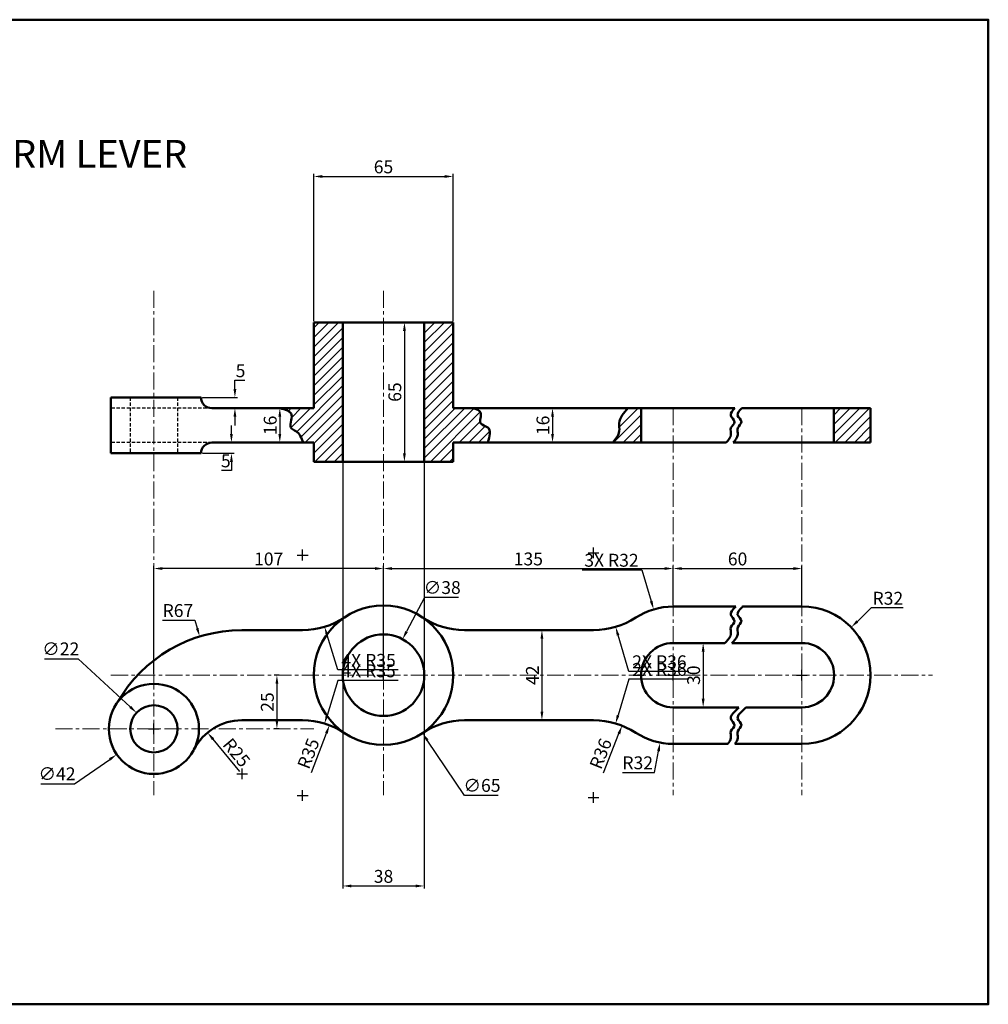
# Model space of a CAD drawing. Units: millimetres. Extents: x -1099 to -222, y 37 to 495.
# Tile 3 of 3: x -674 to -222, y 37 to 495. Entities that reach past the tile are written whole.
import ezdxf

# ---------------------------------------------------------------- set-up
doc = ezdxf.new("R2010")
doc.units = ezdxf.units.MM
doc.header["$LTSCALE"] = 0.5
doc.linetypes.add('CENTER', pattern=[50.8, 31.75, -6.35, 6.35, -6.35])
doc.linetypes.add('HIDDEN', pattern=[9.525, 6.35, -3.175])
for name, color, linetype, lineweight in [('M-CNTR', 1, 'CENTER', 18), ('M-DIMS', 2, 'Continuous', 25), ('M-HATC', 8, 'Continuous', 18), ('M-HIDN', 4, 'HIDDEN', 25), ('M-OUTL', 7, 'Continuous', 50), ('M-TEXT', 7, 'Continuous', 25), ('M-TTLB', 7, 'Continuous', 50)]:
    doc.layers.add(name, color=color, linetype=linetype, lineweight=lineweight)
doc.styles.get("Standard").update_dxf_attribs({"font": 'arial.ttf'})
doc.dimstyles.new('ISO-25', dxfattribs={"dimtxt": 6, "dimasz": 4, "dimexe": 1.25, "dimexo": 0.625, "dimtad": 1, "dimtoh": 1, "dimtxsty": 'Standard', "dimcen": 2.5, "dimadec": 0, "dimazin": 0, "dimtfac": 1, "dimtofl": 0, "dimtmove": 0, "dimatfit": 3, "dimfxl": 1, "dimarcsym": 0})
pattern_1 = [(45, (-1406.9138, -374.9262), (-2.245064, 2.245064), [])]

# ---------------------------------------------------------------- blocks, each defined once
blk = doc.blocks.new('*D20')
at = {"layer": 'Defpoints', "color": 0, "ltscale": 0.5, "transparency": 16777216}
for p in [(-589.05, 319.35), (-573.3, 319.35), (-584.25, 314.35)]:
    blk.add_point(p, dxfattribs=at)
at = {"layer": 'M-DIMS', "color": 0, "lineweight": -2, "ltscale": 0.5, "transparency": 16777216}
for p, q in [((-573.3, 323.35), (-573.3, 327.35)), ((-573.3, 327.35), (-568.69, 327.35)), ((-588.42, 319.35), (-572.05, 319.35)), ((-583.62, 314.35), (-572.05, 314.35)), ((-573.3, 310.35), (-573.3, 306.35))]:
    blk.add_line(p, q, dxfattribs=at)
at = {"layer": 'M-DIMS', "color": 0, "ltscale": 0.5, "transparency": 16777216}
for points in [[(-573.96, 323.35), (-572.63, 323.35), (-573.3, 319.35)], [(-573.96, 310.35), (-572.63, 310.35), (-573.3, 314.35)]]:
    blk.add_solid(points, dxfattribs=at)
at = {"layer": 'M-DIMS', "color": 0, "ltscale": 0.5, "transparency": 16777216, "insert": (-570.68, 331.02), "char_height": 6, "attachment_point": 5}
blk.add_mtext('5', dxfattribs=at)
blk = doc.blocks.new('*D21')
at = {"layer": 'Defpoints', "color": 0, "ltscale": 0.5, "transparency": 16777216}
for p in [(-584.05, 298.35), (-574.92, 298.35), (-589.05, 293.35)]:
    blk.add_point(p, dxfattribs=at)
at = {"layer": 'M-DIMS', "color": 0, "lineweight": -2, "ltscale": 0.5, "transparency": 16777216}
for p, q in [((-574.92, 302.35), (-574.92, 306.35)), ((-583.42, 298.35), (-573.67, 298.35)), ((-588.42, 293.35), (-573.67, 293.35)), ((-574.92, 289.35), (-574.92, 285.35)), ((-574.92, 285.35), (-579.52, 285.35))]:
    blk.add_line(p, q, dxfattribs=at)
at = {"layer": 'M-DIMS', "color": 0, "ltscale": 0.5, "transparency": 16777216}
for points in [[(-575.58, 302.35), (-574.25, 302.35), (-574.92, 298.35)], [(-575.58, 289.35), (-574.25, 289.35), (-574.92, 293.35)]]:
    blk.add_solid(points, dxfattribs=at)
at = {"layer": 'M-DIMS', "color": 0, "ltscale": 0.5, "transparency": 16777216, "insert": (-577.53, 289.02), "char_height": 6, "attachment_point": 5}
blk.add_mtext('5', dxfattribs=at)
blk = doc.blocks.new('*D22')
at = {"layer": 'Defpoints', "color": 0, "ltscale": 0.5, "transparency": 16777216}
for p in [(-552.38, 314.35), (-552.38, 298.35), (-552.38, 298.35)]:
    blk.add_point(p, dxfattribs=at)
at = {"layer": 'M-DIMS', "color": 0, "lineweight": -2, "ltscale": 0.5, "transparency": 16777216}
for p, q in [((-553.01, 314.35), (-553.63, 314.35)), ((-552.38, 310.35), (-552.38, 302.35)), ((-553.01, 298.35), (-553.63, 298.35))]:
    blk.add_line(p, q, dxfattribs=at)
at = {"layer": 'M-DIMS', "color": 0, "ltscale": 0.5, "transparency": 16777216}
for points in [[(-553.05, 310.35), (-551.72, 310.35), (-552.38, 314.35)], [(-553.05, 302.35), (-551.72, 302.35), (-552.38, 298.35)]]:
    blk.add_solid(points, dxfattribs=at)
at = {"layer": 'M-DIMS', "color": 0, "ltscale": 0.5, "transparency": 16777216, "insert": (-556.07, 306.35), "char_height": 6, "attachment_point": 5, "rotation": 90}
blk.add_mtext('16', dxfattribs=at)
blk = doc.blocks.new('*D23')
at = {"layer": 'Defpoints', "color": 0, "ltscale": 0.5, "transparency": 16777216}
for p in [(-495.11, 354.35), (-495.11, 289.35), (-494.3, 289.35)]:
    blk.add_point(p, dxfattribs=at)
at = {"layer": 'M-DIMS', "color": 0, "lineweight": -2, "ltscale": 0.5, "transparency": 16777216}
for p, q in [((-494.48, 354.35), (-493.05, 354.35)), ((-494.3, 350.35), (-494.3, 293.35)), ((-494.48, 289.35), (-493.05, 289.35))]:
    blk.add_line(p, q, dxfattribs=at)
at = {"layer": 'M-DIMS', "color": 0, "ltscale": 0.5, "transparency": 16777216}
for points in [[(-494.97, 350.35), (-493.64, 350.35), (-494.3, 354.35)], [(-494.97, 293.35), (-493.64, 293.35), (-494.3, 289.35)]]:
    blk.add_solid(points, dxfattribs=at)
at = {"layer": 'M-DIMS', "color": 0, "ltscale": 0.5, "transparency": 16777216, "insert": (-497.99, 321.85), "char_height": 6, "attachment_point": 5, "rotation": 90}
blk.add_mtext('65', dxfattribs=at)
blk = doc.blocks.new('*D24')
at = {"layer": 'Defpoints', "color": 0, "ltscale": 0.5, "transparency": 16777216}
for p in [(-423.41, 314.35), (-425.28, 298.35), (-423.41, 298.35)]:
    blk.add_point(p, dxfattribs=at)
at = {"layer": 'M-DIMS', "color": 0, "lineweight": -2, "ltscale": 0.5, "transparency": 16777216}
for p, q in [((-424.04, 314.35), (-426.53, 314.35)), ((-425.28, 310.35), (-425.28, 302.35)), ((-424.04, 298.35), (-426.53, 298.35))]:
    blk.add_line(p, q, dxfattribs=at)
at = {"layer": 'M-DIMS', "color": 0, "ltscale": 0.5, "transparency": 16777216}
for points in [[(-425.95, 310.35), (-424.62, 310.35), (-425.28, 314.35)], [(-425.95, 302.35), (-424.62, 302.35), (-425.28, 298.35)]]:
    blk.add_solid(points, dxfattribs=at)
at = {"layer": 'M-DIMS', "color": 0, "ltscale": 0.5, "transparency": 16777216, "insert": (-428.97, 306.35), "char_height": 6, "attachment_point": 5, "rotation": 90}
blk.add_mtext('16', dxfattribs=at)
blk = doc.blocks.new('*D25')
at = {"layer": 'Defpoints', "color": 0, "ltscale": 0.5, "transparency": 16777216}
for p in [(-369.05, 239.63), (-504.05, 222.43), (-369.05, 221.93)]:
    blk.add_point(p, dxfattribs=at)
at = {"layer": 'M-DIMS', "color": 0, "lineweight": -2, "ltscale": 0.5, "transparency": 16777216}
for p, q in [((-504.05, 223.06), (-504.05, 240.88)), ((-500.05, 239.63), (-373.05, 239.63)), ((-369.05, 222.56), (-369.05, 240.88))]:
    blk.add_line(p, q, dxfattribs=at)
at = {"layer": 'M-DIMS', "color": 0, "ltscale": 0.5, "transparency": 16777216}
for points in [[(-500.05, 240.3), (-500.05, 238.96), (-504.05, 239.63)], [(-373.05, 240.3), (-373.05, 238.96), (-369.05, 239.63)]]:
    blk.add_solid(points, dxfattribs=at)
at = {"layer": 'M-DIMS', "color": 0, "ltscale": 0.5, "transparency": 16777216, "insert": (-436.55, 243.32), "char_height": 6, "attachment_point": 5}
blk.add_mtext('135', dxfattribs=at)
blk = doc.blocks.new('*D26')
at = {"layer": 'Defpoints', "color": 0, "ltscale": 0.5, "transparency": 16777216}
for p in [(-309.05, 239.63), (-369.05, 221.93), (-309.05, 221.93)]:
    blk.add_point(p, dxfattribs=at)
at = {"layer": 'M-DIMS', "color": 0, "lineweight": -2, "ltscale": 0.5, "transparency": 16777216}
for p, q in [((-369.05, 222.56), (-369.05, 240.88)), ((-365.05, 239.63), (-313.05, 239.63)), ((-309.05, 222.56), (-309.05, 240.88))]:
    blk.add_line(p, q, dxfattribs=at)
at = {"layer": 'M-DIMS', "color": 0, "ltscale": 0.5, "transparency": 16777216}
for points in [[(-365.05, 240.3), (-365.05, 238.96), (-369.05, 239.63)], [(-313.05, 240.3), (-313.05, 238.96), (-309.05, 239.63)]]:
    blk.add_solid(points, dxfattribs=at)
at = {"layer": 'M-DIMS', "color": 0, "ltscale": 0.5, "transparency": 16777216, "insert": (-339.05, 243.32), "char_height": 6, "attachment_point": 5}
blk.add_mtext('60', dxfattribs=at)
blk = doc.blocks.new('*D27')
at = {"layer": 'Defpoints', "color": 0, "ltscale": 0.5, "transparency": 16777216}
for p in [(-611.05, 239.63), (-611.05, 189.93), (-504.05, 189.93)]:
    blk.add_point(p, dxfattribs=at)
at = {"layer": 'M-DIMS', "color": 0, "lineweight": -2, "ltscale": 0.5, "transparency": 16777216}
for p, q in [((-611.05, 190.56), (-611.05, 240.88)), ((-508.05, 239.63), (-607.05, 239.63)), ((-504.05, 190.56), (-504.05, 240.88))]:
    blk.add_line(p, q, dxfattribs=at)
at = {"layer": 'M-DIMS', "color": 0, "ltscale": 0.5, "transparency": 16777216}
for points in [[(-607.05, 240.3), (-607.05, 238.96), (-611.05, 239.63)], [(-508.05, 240.3), (-508.05, 238.96), (-504.05, 239.63)]]:
    blk.add_solid(points, dxfattribs=at)
at = {"layer": 'M-DIMS', "color": 0, "ltscale": 0.5, "transparency": 16777216, "insert": (-557.55, 243.32), "char_height": 6, "attachment_point": 5}
blk.add_mtext('107', dxfattribs=at)
blk = doc.blocks.new('*D28')
at = {"layer": 'Defpoints', "color": 0, "ltscale": 0.5, "transparency": 16777216}
for p in [(-619.12, 172.4), (-602.97, 157.46)]:
    blk.add_point(p, dxfattribs=at)
at = {"layer": 'M-DIMS', "color": 0, "lineweight": -2, "ltscale": 0.5, "transparency": 16777216}
for p, q in [((-661.99, 197.57), (-646.3, 197.57)), ((-646.3, 197.57), (-622.06, 175.12)), ((-611.05, 162.43), (-611.05, 167.43)), ((-613.55, 164.93), (-608.55, 164.93))]:
    blk.add_line(p, q, dxfattribs=at)
at = {"layer": 'M-DIMS', "color": 0, "ltscale": 0.5, "transparency": 16777216}
blk.add_solid([(-621.6, 175.61), (-622.51, 174.63), (-619.12, 172.4)], dxfattribs=at)
at = {"layer": 'M-DIMS', "color": 0, "ltscale": 0.5, "transparency": 16777216, "insert": (-654.46, 201.42), "char_height": 6, "attachment_point": 5}
blk.add_mtext('∅22', dxfattribs=at)
blk = doc.blocks.new('*D29')
at = {"layer": 'Defpoints', "color": 0, "ltscale": 0.5, "transparency": 16777216}
for p in [(-593.77, 176.87), (-628.32, 152.99)]:
    blk.add_point(p, dxfattribs=at)
at = {"layer": 'M-DIMS', "color": 0, "lineweight": -2, "ltscale": 0.5, "transparency": 16777216}
for p, q in [((-611.05, 162.43), (-611.05, 167.43)), ((-613.55, 164.93), (-608.55, 164.93)), ((-648.03, 139.36), (-631.61, 150.71)), ((-663.72, 139.36), (-648.03, 139.36))]:
    blk.add_line(p, q, dxfattribs=at)
at = {"layer": 'M-DIMS', "color": 0, "ltscale": 0.5, "transparency": 16777216}
blk.add_solid([(-631.99, 151.26), (-631.23, 150.17), (-628.32, 152.99)], dxfattribs=at)
at = {"layer": 'M-DIMS', "color": 0, "ltscale": 0.5, "transparency": 16777216, "insert": (-656.19, 143.22), "char_height": 6, "attachment_point": 5}
blk.add_mtext('∅42', dxfattribs=at)
blk = doc.blocks.new('*D30')
at = {"layer": 'Defpoints', "color": 0, "ltscale": 0.5, "transparency": 16777216}
for p in [(-552.13, 189.93), (-553.72, 164.93), (-552.13, 164.93)]:
    blk.add_point(p, dxfattribs=at)
at = {"layer": 'M-DIMS', "color": 0, "lineweight": -2, "ltscale": 0.5, "transparency": 16777216}
for p, q in [((-552.75, 189.93), (-554.97, 189.93)), ((-553.72, 185.93), (-553.72, 168.93)), ((-552.75, 164.93), (-554.97, 164.93))]:
    blk.add_line(p, q, dxfattribs=at)
at = {"layer": 'M-DIMS', "color": 0, "ltscale": 0.5, "transparency": 16777216}
for points in [[(-554.39, 185.93), (-553.06, 185.93), (-553.72, 189.93)], [(-554.39, 168.93), (-553.06, 168.93), (-553.72, 164.93)]]:
    blk.add_solid(points, dxfattribs=at)
at = {"layer": 'M-DIMS', "color": 0, "ltscale": 0.5, "transparency": 16777216, "insert": (-557.41, 177.43), "char_height": 6, "attachment_point": 5, "rotation": 90}
blk.add_mtext('25', dxfattribs=at)
blk = doc.blocks.new('*D31')
at = {"layer": 'Defpoints', "color": 0, "ltscale": 0.5, "transparency": 16777216}
for p in [(-522.19, 216.89), (-485.9, 162.97)]:
    blk.add_point(p, dxfattribs=at)
at = {"layer": 'M-DIMS', "color": 0, "lineweight": -2, "ltscale": 0.5, "transparency": 16777216}
for p, q in [((-506.55, 189.93), (-501.55, 189.93)), ((-504.05, 187.43), (-504.05, 192.43)), ((-466.36, 133.93), (-483.67, 159.65)), ((-450.57, 133.93), (-466.36, 133.93))]:
    blk.add_line(p, q, dxfattribs=at)
at = {"layer": 'M-DIMS', "color": 0, "ltscale": 0.5, "transparency": 16777216}
blk.add_solid([(-483.12, 160.02), (-484.22, 159.28), (-485.9, 162.97)], dxfattribs=at)
at = {"layer": 'M-DIMS', "color": 0, "ltscale": 0.5, "transparency": 16777216, "insert": (-458.15, 137.79), "char_height": 6, "attachment_point": 5}
blk.add_mtext('∅65', dxfattribs=at)
blk = doc.blocks.new('*D32')
at = {"layer": 'Defpoints', "color": 0, "ltscale": 0.5, "transparency": 16777216}
for p in [(-495.16, 206.72), (-512.93, 173.14)]:
    blk.add_point(p, dxfattribs=at)
at = {"layer": 'M-DIMS', "color": 0, "lineweight": -2, "ltscale": 0.5, "transparency": 16777216}
for p, q in [((-484.88, 226.15), (-493.29, 210.26)), ((-469.12, 226.15), (-484.88, 226.15)), ((-506.55, 189.93), (-501.55, 189.93)), ((-504.05, 187.43), (-504.05, 192.43))]:
    blk.add_line(p, q, dxfattribs=at)
at = {"layer": 'M-DIMS', "color": 0, "ltscale": 0.5, "transparency": 16777216}
blk.add_solid([(-493.88, 210.57), (-492.7, 209.95), (-495.16, 206.72)], dxfattribs=at)
at = {"layer": 'M-DIMS', "color": 0, "ltscale": 0.5, "transparency": 16777216, "insert": (-476.69, 230), "char_height": 6, "attachment_point": 5}
blk.add_mtext('∅38', dxfattribs=at)
blk = doc.blocks.new('*D33')
at = {"layer": 'Defpoints', "color": 0, "ltscale": 0.5, "transparency": 16777216}
for p in [(-436.24, 210.93), (-436.24, 168.93), (-430.23, 168.93)]:
    blk.add_point(p, dxfattribs=at)
at = {"layer": 'M-DIMS', "color": 0, "lineweight": -2, "ltscale": 0.5, "transparency": 16777216}
for p, q in [((-435.62, 210.93), (-428.98, 210.93)), ((-430.23, 206.93), (-430.23, 172.93)), ((-435.62, 168.93), (-428.98, 168.93))]:
    blk.add_line(p, q, dxfattribs=at)
at = {"layer": 'M-DIMS', "color": 0, "ltscale": 0.5, "transparency": 16777216}
for points in [[(-430.9, 206.93), (-429.56, 206.93), (-430.23, 210.93)], [(-430.9, 172.93), (-429.56, 172.93), (-430.23, 168.93)]]:
    blk.add_solid(points, dxfattribs=at)
at = {"layer": 'M-DIMS', "color": 0, "ltscale": 0.5, "transparency": 16777216, "insert": (-433.87, 189.93), "char_height": 6, "attachment_point": 5, "rotation": 90}
blk.add_mtext('42', dxfattribs=at)
blk = doc.blocks.new('*D34')
at = {"layer": 'Defpoints', "color": 0, "ltscale": 0.5, "transparency": 16777216}
for p in [(-360.49, 204.93), (-360.49, 174.93), (-355.09, 174.93)]:
    blk.add_point(p, dxfattribs=at)
at = {"layer": 'M-DIMS', "color": 0, "lineweight": -2, "ltscale": 0.5, "transparency": 16777216}
for p, q in [((-359.87, 204.93), (-353.84, 204.93)), ((-355.09, 200.93), (-355.09, 178.93)), ((-359.87, 174.93), (-353.84, 174.93))]:
    blk.add_line(p, q, dxfattribs=at)
at = {"layer": 'M-DIMS', "color": 0, "ltscale": 0.5, "transparency": 16777216}
for points in [[(-355.75, 200.93), (-354.42, 200.93), (-355.09, 204.93)], [(-355.75, 178.93), (-354.42, 178.93), (-355.09, 174.93)]]:
    blk.add_solid(points, dxfattribs=at)
at = {"layer": 'M-DIMS', "color": 0, "ltscale": 0.5, "transparency": 16777216, "insert": (-358.78, 189.93), "char_height": 6, "attachment_point": 5, "rotation": 90}
blk.add_mtext('30', dxfattribs=at)
blk = doc.blocks.new('*D37')
at = {"layer": 'Defpoints', "color": 0, "ltscale": 0.5, "transparency": 16777216}
for p in [(-589.7, 207.95), (-569.93, 143.93)]:
    blk.add_point(p, dxfattribs=at)
at = {"layer": 'M-DIMS', "color": 0, "lineweight": -2, "ltscale": 0.5, "transparency": 16777216}
for p, q in [((-607.02, 215.59), (-592.05, 215.59)), ((-592.05, 215.59), (-590.87, 211.77)), ((-572.43, 143.93), (-567.43, 143.93)), ((-569.93, 141.43), (-569.93, 146.43))]:
    blk.add_line(p, q, dxfattribs=at)
at = {"layer": 'M-DIMS', "color": 0, "ltscale": 0.5, "transparency": 16777216}
blk.add_solid([(-590.24, 211.97), (-591.51, 211.58), (-589.7, 207.95)], dxfattribs=at)
at = {"layer": 'M-DIMS', "color": 0, "ltscale": 0.5, "transparency": 16777216, "insert": (-599.85, 219.28), "char_height": 6, "attachment_point": 5}
blk.add_mtext('R67', dxfattribs=at)
blk = doc.blocks.new('*D38')
at = {"layer": 'Defpoints', "color": 0, "ltscale": 0.5, "transparency": 16777216}
for p in [(-529.24, 166.62), (-541.73, 133.93)]:
    blk.add_point(p, dxfattribs=at)
at = {"layer": 'M-DIMS', "color": 0, "lineweight": -2, "ltscale": 0.5, "transparency": 16777216}
blk.add_line((-537.68, 144.55), (-530.67, 162.89), dxfattribs=at)
at = {"layer": 'M-DIMS', "color": 0, "ltscale": 0.5, "transparency": 16777216}
blk.add_solid([(-531.29, 163.13), (-530.04, 162.65), (-529.24, 166.62)], dxfattribs=at)
at = {"layer": 'M-DIMS', "color": 0, "ltscale": 0.5, "transparency": 16777216, "insert": (-538.33, 153.17), "char_height": 6, "attachment_point": 5, "rotation": 69.0844}
blk.add_mtext('R35', dxfattribs=at)
blk = doc.blocks.new('*D39')
at = {"layer": 'Defpoints', "color": 0, "ltscale": 0.5, "transparency": 16777216}
for p in [(-586.05, 163.2), (-570.12, 143.93)]:
    blk.add_point(p, dxfattribs=at)
at = {"layer": 'M-DIMS', "color": 0, "lineweight": -2, "ltscale": 0.5, "transparency": 16777216}
blk.add_line((-570.99, 144.99), (-583.5, 160.11), dxfattribs=at)
at = {"layer": 'M-DIMS', "color": 0, "ltscale": 0.5, "transparency": 16777216}
blk.add_solid([(-582.99, 160.54), (-584.02, 159.69), (-586.05, 163.2)], dxfattribs=at)
at = {"layer": 'M-DIMS', "color": 0, "ltscale": 0.5, "transparency": 16777216, "insert": (-573.13, 153.36), "char_height": 6, "attachment_point": 5, "rotation": 309.587}
blk.add_mtext('R25', dxfattribs=at)
blk = doc.blocks.new('*D40')
at = {"layer": 'Defpoints', "color": 0, "ltscale": 0.5, "transparency": 16777216}
for p in [(-392.89, 166.41), (-406.13, 132.93)]:
    blk.add_point(p, dxfattribs=at)
at = {"layer": 'M-DIMS', "color": 0, "lineweight": -2, "ltscale": 0.5, "transparency": 16777216}
blk.add_line((-401.56, 144.48), (-394.36, 162.69), dxfattribs=at)
at = {"layer": 'M-DIMS', "color": 0, "ltscale": 0.5, "transparency": 16777216}
blk.add_solid([(-394.98, 162.93), (-393.74, 162.44), (-392.89, 166.41)], dxfattribs=at)
at = {"layer": 'M-DIMS', "color": 0, "ltscale": 0.5, "transparency": 16777216, "insert": (-402.13, 153.08), "char_height": 6, "attachment_point": 5, "rotation": 68.4271}
blk.add_mtext('R36', dxfattribs=at)
blk = doc.blocks.new('*D41')
at = {"layer": 'Defpoints', "color": 0, "ltscale": 0.5, "transparency": 16777216}
for p in [(-369.05, 189.93), (-375.14, 158.52)]:
    blk.add_point(p, dxfattribs=at)
at = {"layer": 'M-DIMS', "color": 0, "lineweight": -2, "ltscale": 0.5, "transparency": 16777216}
for p, q in [((-371.55, 189.93), (-366.55, 189.93)), ((-369.05, 187.43), (-369.05, 192.43)), ((-377.83, 144.64), (-375.9, 154.59)), ((-392.73, 144.64), (-377.83, 144.64))]:
    blk.add_line(p, q, dxfattribs=at)
at = {"layer": 'M-DIMS', "color": 0, "ltscale": 0.5, "transparency": 16777216}
blk.add_solid([(-376.55, 154.72), (-375.24, 154.46), (-375.14, 158.52)], dxfattribs=at)
at = {"layer": 'M-DIMS', "color": 0, "ltscale": 0.5, "transparency": 16777216, "insert": (-385.59, 148.33), "char_height": 6, "attachment_point": 5}
blk.add_mtext('R32', dxfattribs=at)
blk = doc.blocks.new('*D42')
at = {"layer": 'Defpoints', "color": 0, "ltscale": 0.5, "transparency": 16777216}
for p in [(-286.1, 212.24), (-309.05, 189.93)]:
    blk.add_point(p, dxfattribs=at)
at = {"layer": 'M-DIMS', "color": 0, "lineweight": -2, "ltscale": 0.5, "transparency": 16777216}
for p, q in [((-276.77, 221.31), (-283.24, 215.03)), ((-261.87, 221.31), (-276.77, 221.31)), ((-311.55, 189.93), (-306.55, 189.93)), ((-309.05, 187.43), (-309.05, 192.43))]:
    blk.add_line(p, q, dxfattribs=at)
at = {"layer": 'M-DIMS', "color": 0, "ltscale": 0.5, "transparency": 16777216}
blk.add_solid([(-283.7, 215.5), (-282.77, 214.55), (-286.1, 212.24)], dxfattribs=at)
at = {"layer": 'M-DIMS', "color": 0, "ltscale": 0.5, "transparency": 16777216, "insert": (-269.01, 225), "char_height": 6, "attachment_point": 5}
blk.add_mtext('R32', dxfattribs=at)
blk = doc.blocks.new('*D43')
at = {"layer": 'Defpoints', "color": 0, "ltscale": 0.5, "transparency": 16777216}
for p in [(-531.52, 167.41), (-541.73, 133.93)]:
    blk.add_point(p, dxfattribs=at)
at = {"layer": 'M-DIMS', "color": 0, "lineweight": -2, "ltscale": 0.5, "transparency": 16777216}
for p, q in [((-525.39, 187.49), (-530.35, 171.23)), ((-497.25, 187.49), (-525.39, 187.49)), ((-544.23, 133.93), (-539.23, 133.93)), ((-541.73, 131.43), (-541.73, 136.43))]:
    blk.add_line(p, q, dxfattribs=at)
at = {"layer": 'M-DIMS', "color": 0, "ltscale": 0.5, "transparency": 16777216}
blk.add_solid([(-530.99, 171.43), (-529.71, 171.04), (-531.52, 167.41)], dxfattribs=at)
at = {"layer": 'M-DIMS', "color": 0, "ltscale": 0.5, "transparency": 16777216, "insert": (-511.01, 191.18), "char_height": 6, "attachment_point": 5}
blk.add_mtext('4X R35', dxfattribs=at)
blk = doc.blocks.new('*D44')
at = {"layer": 'Defpoints', "color": 0, "ltscale": 0.5, "transparency": 16777216}
for p in [(-395.89, 167.44), (-406.13, 132.93)]:
    blk.add_point(p, dxfattribs=at)
at = {"layer": 'M-DIMS', "color": 0, "lineweight": -2, "ltscale": 0.5, "transparency": 16777216}
for p, q in [((-389.75, 188.15), (-394.75, 171.28)), ((-361.79, 188.15), (-389.75, 188.15)), ((-406.13, 130.43), (-406.13, 135.43)), ((-408.63, 132.93), (-403.63, 132.93))]:
    blk.add_line(p, q, dxfattribs=at)
at = {"layer": 'M-DIMS', "color": 0, "ltscale": 0.5, "transparency": 16777216}
blk.add_solid([(-395.39, 171.47), (-394.11, 171.09), (-395.89, 167.44)], dxfattribs=at)
at = {"layer": 'M-DIMS', "color": 0, "ltscale": 0.5, "transparency": 16777216, "insert": (-375.46, 191.84), "char_height": 6, "attachment_point": 5}
blk.add_mtext('2X R36', dxfattribs=at)
blk = doc.blocks.new('*D45')
at = {"layer": 'Defpoints', "color": 0, "ltscale": 0.5, "transparency": 16777216}
for p in [(-471.55, 422.32), (-536.55, 354.35), (-471.55, 354.35)]:
    blk.add_point(p, dxfattribs=at)
at = {"layer": 'M-DIMS', "color": 0, "lineweight": -2, "ltscale": 0.5, "transparency": 16777216}
for p, q in [((-536.55, 354.97), (-536.55, 423.57)), ((-532.55, 422.32), (-475.55, 422.32)), ((-471.55, 354.97), (-471.55, 423.57))]:
    blk.add_line(p, q, dxfattribs=at)
at = {"layer": 'M-DIMS', "color": 0, "ltscale": 0.5, "transparency": 16777216}
for points in [[(-532.55, 422.99), (-532.55, 421.65), (-536.55, 422.32)], [(-475.55, 422.99), (-475.55, 421.65), (-471.55, 422.32)]]:
    blk.add_solid(points, dxfattribs=at)
at = {"layer": 'M-DIMS', "color": 0, "ltscale": 0.5, "transparency": 16777216, "insert": (-504.05, 426.01), "char_height": 6, "attachment_point": 5}
blk.add_mtext('65', dxfattribs=at)
blk = doc.blocks.new('*D46')
at = {"layer": 'Defpoints', "color": 0, "ltscale": 0.5, "transparency": 16777216}
for p in [(-523.05, 289.35), (-485.05, 289.35), (-485.05, 91.72)]:
    blk.add_point(p, dxfattribs=at)
at = {"layer": 'M-DIMS', "color": 0, "lineweight": -2, "ltscale": 0.5, "transparency": 16777216}
for p, q in [((-523.05, 288.72), (-523.05, 90.47)), ((-485.05, 288.72), (-485.05, 90.47)), ((-519.05, 91.72), (-489.05, 91.72))]:
    blk.add_line(p, q, dxfattribs=at)
at = {"layer": 'M-DIMS', "color": 0, "ltscale": 0.5, "transparency": 16777216}
for points in [[(-519.05, 92.38), (-519.05, 91.05), (-523.05, 91.72)], [(-489.05, 92.38), (-489.05, 91.05), (-485.05, 91.72)]]:
    blk.add_solid(points, dxfattribs=at)
at = {"layer": 'M-DIMS', "color": 0, "ltscale": 0.5, "transparency": 16777216, "insert": (-504.05, 95.41), "char_height": 6, "attachment_point": 5}
blk.add_mtext('38', dxfattribs=at)
blk = doc.blocks.new('*D47')
at = {"layer": 'Defpoints', "color": 0, "ltscale": 0.5, "transparency": 16777216}
for p in [(-541.73, 245.93), (-531.52, 212.45)]:
    blk.add_point(p, dxfattribs=at)
at = {"layer": 'M-DIMS', "color": 0, "lineweight": -2, "ltscale": 0.5, "transparency": 16777216}
for p, q in [((-541.73, 243.43), (-541.73, 248.43)), ((-544.23, 245.93), (-539.23, 245.93)), ((-525.39, 192.37), (-530.35, 208.63)), ((-497.25, 192.37), (-525.39, 192.37))]:
    blk.add_line(p, q, dxfattribs=at)
at = {"layer": 'M-DIMS', "color": 0, "ltscale": 0.5, "transparency": 16777216}
blk.add_solid([(-529.71, 208.82), (-530.99, 208.43), (-531.52, 212.45)], dxfattribs=at)
at = {"layer": 'M-DIMS', "color": 0, "ltscale": 0.5, "transparency": 16777216, "insert": (-511.01, 196.06), "char_height": 6, "attachment_point": 5}
blk.add_mtext('4X R35', dxfattribs=at)
blk = doc.blocks.new('*D48')
at = {"layer": 'Defpoints', "color": 0, "ltscale": 0.5, "transparency": 16777216}
for p in [(-406.13, 246.93), (-395.89, 212.42)]:
    blk.add_point(p, dxfattribs=at)
at = {"layer": 'M-DIMS', "color": 0, "lineweight": -2, "ltscale": 0.5, "transparency": 16777216}
for p, q in [((-406.13, 244.43), (-406.13, 249.43)), ((-408.63, 246.93), (-403.63, 246.93)), ((-389.75, 191.71), (-394.75, 208.58)), ((-361.79, 191.71), (-389.75, 191.71))]:
    blk.add_line(p, q, dxfattribs=at)
at = {"layer": 'M-DIMS', "color": 0, "ltscale": 0.5, "transparency": 16777216}
blk.add_solid([(-394.11, 208.77), (-395.39, 208.39), (-395.89, 212.42)], dxfattribs=at)
at = {"layer": 'M-DIMS', "color": 0, "ltscale": 0.5, "transparency": 16777216, "insert": (-375.46, 195.4), "char_height": 6, "attachment_point": 5}
blk.add_mtext('2X R36', dxfattribs=at)
blk = doc.blocks.new('*D50')
at = {"layer": 'Defpoints', "color": 0, "ltscale": 0.5, "transparency": 16777216}
for p in [(-378.15, 220.61), (-369.05, 189.93)]:
    blk.add_point(p, dxfattribs=at)
at = {"layer": 'M-DIMS', "color": 0, "lineweight": -2, "ltscale": 0.5, "transparency": 16777216}
for p, q in [((-411.4, 239.02), (-383.61, 239.02)), ((-383.61, 239.02), (-379.29, 224.44)), ((-371.55, 189.93), (-366.55, 189.93)), ((-369.05, 187.43), (-369.05, 192.43))]:
    blk.add_line(p, q, dxfattribs=at)
at = {"layer": 'M-DIMS', "color": 0, "ltscale": 0.5, "transparency": 16777216}
blk.add_solid([(-378.65, 224.63), (-379.92, 224.25), (-378.15, 220.61)], dxfattribs=at)
at = {"layer": 'M-DIMS', "color": 0, "ltscale": 0.5, "transparency": 16777216, "insert": (-397.82, 242.71), "char_height": 6, "attachment_point": 5}
blk.add_mtext('3X R32', dxfattribs=at)

msp = doc.modelspace()

# ---------------------------------------------------------------- hatches: boundary and pattern name
at = {"layer": 'M-HATC', "ltscale": 0.5}
h = msp.add_hatch(dxfattribs=at)
h.set_pattern_fill('ANSI31', color=256)
h.set_pattern_definition(pattern_1)
edge = h.paths.add_edge_path()
edge.add_line((-523.047, 354.345), (-536.547, 354.345))
edge.add_line((-536.547, 354.345), (-536.547, 314.345))
edge.add_line((-536.547, 314.345), (-552.384, 314.345))
edge.add_spline(control_points=[(-552.384, 314.345), (-549.851, 313.699), (-544.778, 312.406), (-548.765, 305.073), (-543.306, 303.36), (-542.294, 300.475), (-541.546, 298.345)], knot_values=[0, 0, 0, 0, 6.3399626, 12.6922631, 14.9383718, 21.282806, 21.282806, 21.282806, 21.282806], degree=3, periodic=0)
edge.add_line((-541.546, 298.345), (-536.547, 298.345))
edge.add_line((-536.547, 298.345), (-536.547, 289.345))
edge.add_line((-536.547, 289.345), (-523.047, 289.345))
edge.add_line((-523.047, 289.345), (-523.047, 354.345))
edge = h.paths.add_edge_path()
edge.add_spline(control_points=[(-455.505, 298.345), (-454.606, 301.216), (-453.23, 305.608), (-460.389, 306.69), (-457.243, 312.852), (-460.861, 313.862), (-462.59, 314.345)], knot_values=[0, 0, 0, 0, 7.0551046, 10.792213, 15.6466829, 20.0904255, 20.0904255, 20.0904255, 20.0904255], degree=3, periodic=0)
edge.add_line((-462.59, 314.345), (-471.547, 314.345))
edge.add_line((-471.547, 314.345), (-471.547, 354.345))
edge.add_line((-471.547, 354.345), (-485.047, 354.345))
edge.add_line((-485.047, 354.345), (-485.047, 289.345))
edge.add_line((-485.047, 289.345), (-471.547, 289.345))
edge.add_line((-471.547, 289.345), (-471.547, 298.345))
edge.add_line((-471.547, 298.345), (-455.505, 298.345))
edge = h.paths.add_edge_path()
edge.add_line((-903.92, 354.345), (-915.42, 354.345))
edge.add_line((-915.42, 354.345), (-915.42, 307.345))
edge.add_line((-915.42, 307.345), (-896.253, 307.345))
edge.add_spline(control_points=[(-896.253, 307.345), (-895.98, 308.452), (-896.888, 311.207), (-895.167, 313.257), (-894.255, 314.345)], knot_values=[0, 0, 0, 0, 3.5385178, 7.5354932, 7.5354932, 7.5354932, 7.5354932], degree=3, periodic=0)
edge.add_line((-894.255, 314.345), (-903.92, 314.345))
edge.add_line((-903.92, 314.345), (-903.92, 354.345))
edge = h.paths.add_edge_path()
edge.add_spline(control_points=[(-898.387, 300.345), (-898.564, 301.494), (-898.971, 304.127), (-896.582, 306.011), (-896.253, 307.345)], knot_values=[7.5354932, 7.5354932, 7.5354932, 7.5354932, 10.8396757, 15.1072381, 15.1072381, 15.1072381, 15.1072381], degree=3, periodic=0)
edge.add_line((-896.253, 307.345), (-915.42, 307.345))
edge.add_line((-915.42, 307.345), (-915.42, 300.345))
edge.add_line((-915.42, 300.345), (-898.387, 300.345))
h = msp.add_hatch(dxfattribs=at)
h.set_pattern_fill('ANSI31', color=256)
h.set_pattern_definition(pattern_1)
edge = h.paths.add_edge_path()
edge.add_line((-384.047, 314.345), (-390.163, 314.345))
edge.add_spline(control_points=[(-390.163, 314.345), (-392.069, 312.168), (-394.872, 308.967), (-393.597, 302.663), (-395.837, 299.988), (-397.212, 298.345)], knot_values=[0, 0, 0, 0, 8.0645322, 11.8544893, 17.8889002, 17.8889002, 17.8889002, 17.8889002], degree=3, periodic=0)
edge.add_line((-397.212, 298.345), (-384.047, 298.345))
edge.add_line((-384.047, 298.345), (-384.047, 314.345))
h.paths.add_polyline_path([(-277.047, 314.345), (-294.26, 314.345), (-294.26, 298.345), (-277.047, 298.345)])

# ---------------------------------------------------------------- linework, layer by layer
at = {"layer": 'M-CNTR', "ltscale": 0.5}
for p, q in [((-611.047, 369.083), (-611.047, 134.066)), ((-504.047, 369.083), (-504.047, 134.066)), ((-369.047, 314.345), (-369.047, 134.066)), ((-309.047, 314.345), (-309.047, 134.066)), ((-631.047, 189.931), (-248.287, 189.931)), ((-656.971, 164.931), (-536.547, 164.931))]:
    msp.add_line(p, q, dxfattribs=at)
at = {"layer": 'M-HIDN', "ltscale": 0.5}
for p, q in [((-622.047, 319.345), (-622.047, 293.345)), ((-600.047, 319.345), (-600.047, 293.345)), ((-584.047, 314.345), (-631.047, 314.345)), ((-584.047, 298.345), (-631.047, 298.345))]:
    msp.add_line(p, q, dxfattribs=at)
at = {"layer": 'M-OUTL'}
for p, q in [((-536.547, 354.345), (-471.547, 354.345)), ((-536.547, 314.345), (-536.547, 354.345)), ((-471.547, 314.345), (-471.547, 354.345)), ((-631.047, 319.345), (-631.047, 293.345)), ((-584.047, 314.345), (-536.547, 314.345)), ((-471.547, 314.345), (-340.296, 314.345)), ((-337.082, 314.345), (-277.047, 314.345)), ((-584.047, 298.345), (-536.547, 298.345)), ((-536.547, 289.345), (-536.547, 298.345)), ((-471.547, 289.345), (-471.547, 298.345)), ((-471.547, 298.345), (-344.387, 298.345)), ((-341.173, 298.345), (-277.047, 298.345)), ((-536.547, 289.345), (-471.547, 289.345))]:
    msp.add_line(p, q, dxfattribs=at)
at = {"layer": 'M-OUTL', "ltscale": 0.5}
for p, q in [((-523.047, 354.345), (-523.047, 289.345)), ((-485.047, 354.345), (-485.047, 289.345)), ((-631.047, 319.345), (-589.047, 319.345)), ((-589.047, 319.345), (-589.047, 319.345)), ((-384.047, 298.345), (-384.047, 314.345)), ((-294.26, 298.345), (-294.26, 314.345)), ((-277.047, 298.345), (-277.047, 314.345)), ((-631.047, 293.345), (-589.047, 293.345)), ((-589.047, 293.345), (-589.047, 293.345)), ((-369.047, 221.931), (-339.849, 221.931)), ((-336.635, 221.931), (-309.047, 221.931)), ((-570.12, 210.931), (-541.733, 210.931)), ((-466.361, 210.931), (-406.128, 210.931)), ((-344.916, 204.931), (-369.047, 204.931)), ((-309.047, 204.931), (-341.702, 204.931)), ((-369.047, 174.931), (-338.413, 174.931)), ((-335.2, 174.931), (-309.047, 174.931)), ((-570.12, 168.931), (-541.733, 168.931)), ((-466.361, 168.931), (-406.128, 168.931)), ((-369.047, 157.931), (-343.589, 157.931)), ((-340.376, 157.931), (-309.047, 157.931))]:
    msp.add_line(p, q, dxfattribs=at)
for centre, radius in [((-504.047, 189.931), 32.5), ((-504.047, 189.931), 19), ((-611.047, 164.931), 21), ((-611.047, 164.931), 11)]:
    msp.add_circle(centre, radius, dxfattribs=at)
at = {"layer": 'M-OUTL'}
for centre, start, end in [((-584.047, 319.345), 180, 270), ((-584.047, 293.345), 90, 180)]:
    msp.add_arc(centre, 5, start, end, dxfattribs=at)
at = {"layer": 'M-OUTL', "ltscale": 0.5}
for centre, radius, start, end in [((-369.047, 189.931), 32, 90, 123.04576), ((-309.047, 189.931), 32, 270, 90), ((-541.733, 245.931), 35, 270, 303.93929), ((-466.361, 245.931), 35, 236.06071, 270), ((-406.128, 246.931), 36, 270, 303.04576), ((-569.934, 143.931), 67, 90.15966, 150.22754), ((-369.047, 189.931), 15, 90, 270), ((-309.047, 189.931), 15, 270, 90), ((-570.12, 143.931), 25, 90, 152.83711), ((-541.733, 133.931), 35, 56.06071, 90), ((-466.361, 133.931), 35, 90, 123.93929), ((-406.128, 132.931), 36, 56.95424, 90), ((-369.047, 189.931), 32, 236.95424, 270)]:
    msp.add_arc(centre, radius, start, end, dxfattribs=at)
for points, knots in [([(-552.384, 314.345), (-549.851, 313.699), (-544.778, 312.406), (-548.765, 305.073), (-543.306, 303.36), (-542.294, 300.475), (-541.546, 298.345)], [0, 0, 0, 0, 6.3399626, 12.6922631, 14.9383718, 21.282806, 21.282806, 21.282806, 21.282806]), ([(-462.59, 314.345), (-460.861, 313.862), (-457.243, 312.852), (-460.389, 306.69), (-453.23, 305.608), (-454.606, 301.216), (-455.505, 298.345)], [0, 0, 0, 0, 4.4437426, 9.2982125, 13.0353208, 20.0904255, 20.0904255, 20.0904255, 20.0904255]), ([(-397.212, 298.345), (-395.837, 299.988), (-393.597, 302.663), (-394.872, 308.967), (-392.069, 312.168), (-390.163, 314.345)], [0, 0, 0, 0, 6.0344109, 9.824368, 17.8889002, 17.8889002, 17.8889002, 17.8889002]), ([(-340.296, 314.345), (-341.421, 313.232), (-343.556, 311.119), (-339.136, 307.985), (-342.989, 305.315), (-341.464, 301.428), (-343.322, 299.468), (-344.387, 298.345)], [0, 0, 0, 0, 3.873202, 7.3473783, 10.65582, 13.8203852, 18.0651949, 18.0651949, 18.0651949, 18.0651949]), ([(-337.082, 314.345), (-338.208, 313.232), (-340.343, 311.119), (-335.923, 307.985), (-339.776, 305.315), (-338.251, 301.428), (-340.109, 299.468), (-341.173, 298.345)], [0, 0, 0, 0, 3.873202, 7.3473783, 10.65582, 13.8203852, 18.0651949, 18.0651949, 18.0651949, 18.0651949]), ([(-339.849, 221.931), (-339.998, 221.784), (-340.147, 221.636), (-340.296, 221.489), (-341.421, 220.375), (-343.556, 218.263), (-339.136, 215.129), (-342.989, 212.458), (-341.464, 208.572), (-343.322, 206.612), (-344.387, 205.489), (-344.563, 205.303), (-344.739, 205.117), (-344.916, 204.931)], [-0.51263, -0.51263, -0.51263, -0.51263, 0, 0, 0, 3.873202, 7.3473783, 10.65582, 13.8203852, 18.0651949, 18.0651949, 18.0651949, 18.7681141, 18.7681141, 18.7681141, 18.7681141]), ([(-336.635, 221.931), (-336.784, 221.784), (-336.933, 221.636), (-337.082, 221.489), (-338.208, 220.375), (-340.343, 218.263), (-335.923, 215.129), (-339.776, 212.458), (-338.251, 208.572), (-340.109, 206.612), (-341.173, 205.489), (-341.35, 205.303), (-341.526, 205.117), (-341.702, 204.931)], [-0.51263, -0.51263, -0.51263, -0.51263, 0, 0, 0, 3.873202, 7.3473783, 10.65582, 13.8203852, 18.0651949, 18.0651949, 18.0651949, 18.7681141, 18.7681141, 18.7681141, 18.7681141]), ([(-338.413, 174.931), (-339.041, 174.31), (-339.668, 173.689), (-340.296, 173.069), (-341.421, 171.955), (-343.556, 169.843), (-339.136, 166.709), (-342.989, 164.038), (-341.618, 160.544), (-342.842, 158.779), (-343.589, 157.931)], [-2.1589222, -2.1589222, -2.1589222, -2.1589222, 0, 0, 0, 3.873202, 7.3473783, 10.65582, 13.8203852, 16.983683, 16.983683, 16.983683, 16.983683]), ([(-335.2, 174.931), (-335.827, 174.31), (-336.455, 173.689), (-337.082, 173.069), (-338.208, 171.955), (-340.343, 169.843), (-335.923, 166.709), (-339.776, 164.038), (-338.405, 160.544), (-339.629, 158.779), (-340.376, 157.931)], [-2.1589222, -2.1589222, -2.1589222, -2.1589222, 0, 0, 0, 3.873202, 7.3473783, 10.65582, 13.8203852, 16.983683, 16.983683, 16.983683, 16.983683])]:
    msp.add_open_spline(points, degree=3, knots=knots, dxfattribs=at)
at = {"layer": 'M-TTLB', "ltscale": 0.5}
msp.add_lwpolyline([(-1099.005, 495.37), (-222.205, 495.37), (-222.205, 36.581), (-1099.005, 36.581)], close=True, dxfattribs=at)

# ---------------------------------------------------------------- texts
at = {"layer": 'M-TEXT', "ltscale": 0.5, "insert": (-761.792, 439.344), "char_height": 13, "attachment_point": 1}
msp.add_mtext_dynamic_manual_height_columns('DOUBLE ARM LEVER', width=201.89574, gutter_width=12.5, heights=[0], dxfattribs=at)

# ---------------------------------------------------------------- dimensions: what is measured, and where the dimension line sits
at = {"layer": 'M-DIMS', "ltscale": 0.5}
for base, p1, p2, override, picture, middle in [((-471.547, 422.319), (-536.547, 354.345), (-471.547, 354.345), {"dimdec": 0, "dimlfac": 1, "dimrnd": 0, "dimzin": 0, "dimdsep": 46, "dimlunit": 2}, '*D45', (-504.047, 426.008)), ((-485.047, 91.716), (-523.047, 289.345), (-485.047, 289.345), {"dimdec": 0, "dimlfac": 1, "dimrnd": 0, "dimzin": 0, "dimdsep": 46, "dimlunit": 2}, '*D46', (-504.047, 95.406)), ((-611.047, 239.631), (-504.047, 189.931), (-611.047, 189.931), {"dimclrd": 0, "dimclre": 0, "dimclrt": 0}, '*D27', (-557.547, 243.32)), ((-369.047, 239.631), (-504.047, 222.431), (-369.047, 221.931), {"dimclrd": 0, "dimclre": 0, "dimclrt": 0}, '*D25', (-436.547, 243.322)), ((-309.047, 239.631), (-369.047, 221.931), (-309.047, 221.931), {"dimclrd": 0, "dimclre": 0, "dimclrt": 0}, '*D26', (-339.047, 243.32))]:
    dim = msp.add_linear_dim(base=base, p1=p1, p2=p2, dimstyle='ISO-25', override=override, dxfattribs=at)
    dim.commit()
    dim.dimension.update_dxf_attribs({"geometry": picture, "text_midpoint": middle})
for base, p1, p2, picture, middle in [((-494.303, 289.345), (-495.108, 354.345), (-495.108, 289.345), '*D23', (-497.992, 321.845)), ((-573.296, 319.345), (-584.248, 314.349), (-589.047, 319.345), '*D20', (-570.682, 331.021)), ((-552.384, 298.345), (-552.384, 314.345), (-552.384, 298.345), '*D22', (-556.073, 306.345)), ((-425.282, 298.345), (-423.412, 314.345), (-423.412, 298.345), '*D24', (-428.97, 306.345)), ((-430.232, 168.931), (-436.245, 210.931), (-436.245, 168.931), '*D33', (-433.869, 189.931)), ((-355.087, 174.931), (-360.493, 204.931), (-360.493, 174.931), '*D34', (-358.778, 189.931)), ((-553.724, 164.931), (-552.129, 189.931), (-552.129, 164.931), '*D30', (-557.412, 177.431))]:
    dim = msp.add_linear_dim(base=base, p1=p1, p2=p2, angle=90, dimstyle='ISO-25', override={"dimclrd": 0, "dimclre": 0, "dimclrt": 0}, dxfattribs=at)
    dim.commit()
    dim.dimension.update_dxf_attribs({"geometry": picture, "text_midpoint": middle})
dim = msp.add_linear_dim(base=(-574.918, 298.345), p1=(-589.047, 293.345), p2=(-584.047, 298.345), angle=90, dimstyle='ISO-25', override={"dimclrd": 0, "dimclre": 0, "dimclrt": 0}, dxfattribs=at)
dim.commit()
dim.dimension.update_dxf_attribs({"geometry": '*D21', "text_midpoint": (-577.532, 285.345), "dimtype": 160})
for center, mpoint, text, picture, middle in [((-541.733, 245.931), (-531.52, 212.454), '4X <>', '*D47', (-511.009, 192.368)), ((-369.047, 189.931), (-378.148, 220.61), '3X <>', '*D50', (-397.815, 239.017)), ((-406.128, 246.931), (-395.89, 212.418), '2X <>', '*D48', (-375.458, 191.709)), ((-541.733, 133.931), (-531.518, 167.407), '4X <>', '*D43', (-511.006, 187.493)), ((-406.128, 132.931), (-395.889, 167.444), '2X <>', '*D44', (-375.456, 188.152))]:
    dim = msp.add_radius_dim(center=center, mpoint=mpoint, text=text, dimstyle='ISO-25', override={"dimdec": 0, "dimlfac": 1, "dimrnd": 0, "dimzin": 0, "dimdsep": 46, "dimlunit": 2}, dxfattribs=at)
    dim.commit()
    dim.dimension.update_dxf_attribs({"geometry": picture, "text_midpoint": middle, "dimtype": 164})
for p1, p2, picture, middle in [((-512.935, 173.138), (-495.159, 206.724), '*D32', (-476.687, 226.148)), ((-522.192, 216.894), (-485.902, 162.968), '*D31', (-458.152, 133.931)), ((-602.975, 157.459), (-619.12, 172.403), '*D28', (-654.459, 197.565)), ((-593.773, 176.873), (-628.321, 152.989), '*D29', (-656.189, 139.362))]:
    dim = msp.add_diameter_dim_2p(p1=p1, p2=p2, dimstyle='ISO-25', override={"dimclrd": 0, "dimclre": 0, "dimclrt": 0}, dxfattribs=at)
    dim.commit()
    dim.dimension.update_dxf_attribs({"geometry": picture, "text_midpoint": middle, "dimtype": 163})
for center, mpoint, picture, middle in [((-309.047, 189.931), (-286.104, 212.238), '*D42', (-269.01, 221.31)), ((-541.733, 133.931), (-529.239, 166.625), '*D38', (-534.885, 151.851)), ((-406.128, 132.931), (-392.892, 166.409), '*D40', (-398.698, 151.724)), ((-570.12, 143.931), (-586.052, 163.197), '*D39', (-575.973, 151.009))]:
    dim = msp.add_radius_dim(center=center, mpoint=mpoint, dimstyle='ISO-25', override={"dimclrd": 0, "dimclre": 0, "dimclrt": 0}, dxfattribs=at)
    dim.commit()
    dim.dimension.update_dxf_attribs({"geometry": picture, "text_midpoint": middle, "dimtype": 164})
for center, mpoint, picture, middle in [((-569.934, 143.931), (-589.695, 207.951), '*D37', (-599.848, 219.283)), ((-369.047, 189.931), (-375.138, 158.516), '*D41', (-385.59, 148.334))]:
    dim = msp.add_radius_dim(center=center, mpoint=mpoint, dimstyle='ISO-25', override={"dimclrd": 0, "dimclre": 0, "dimclrt": 0}, dxfattribs=at)
    dim.commit()
    dim.dimension.update_dxf_attribs({"geometry": picture, "text_midpoint": middle})

doc.saveas('drawing.dxf')
